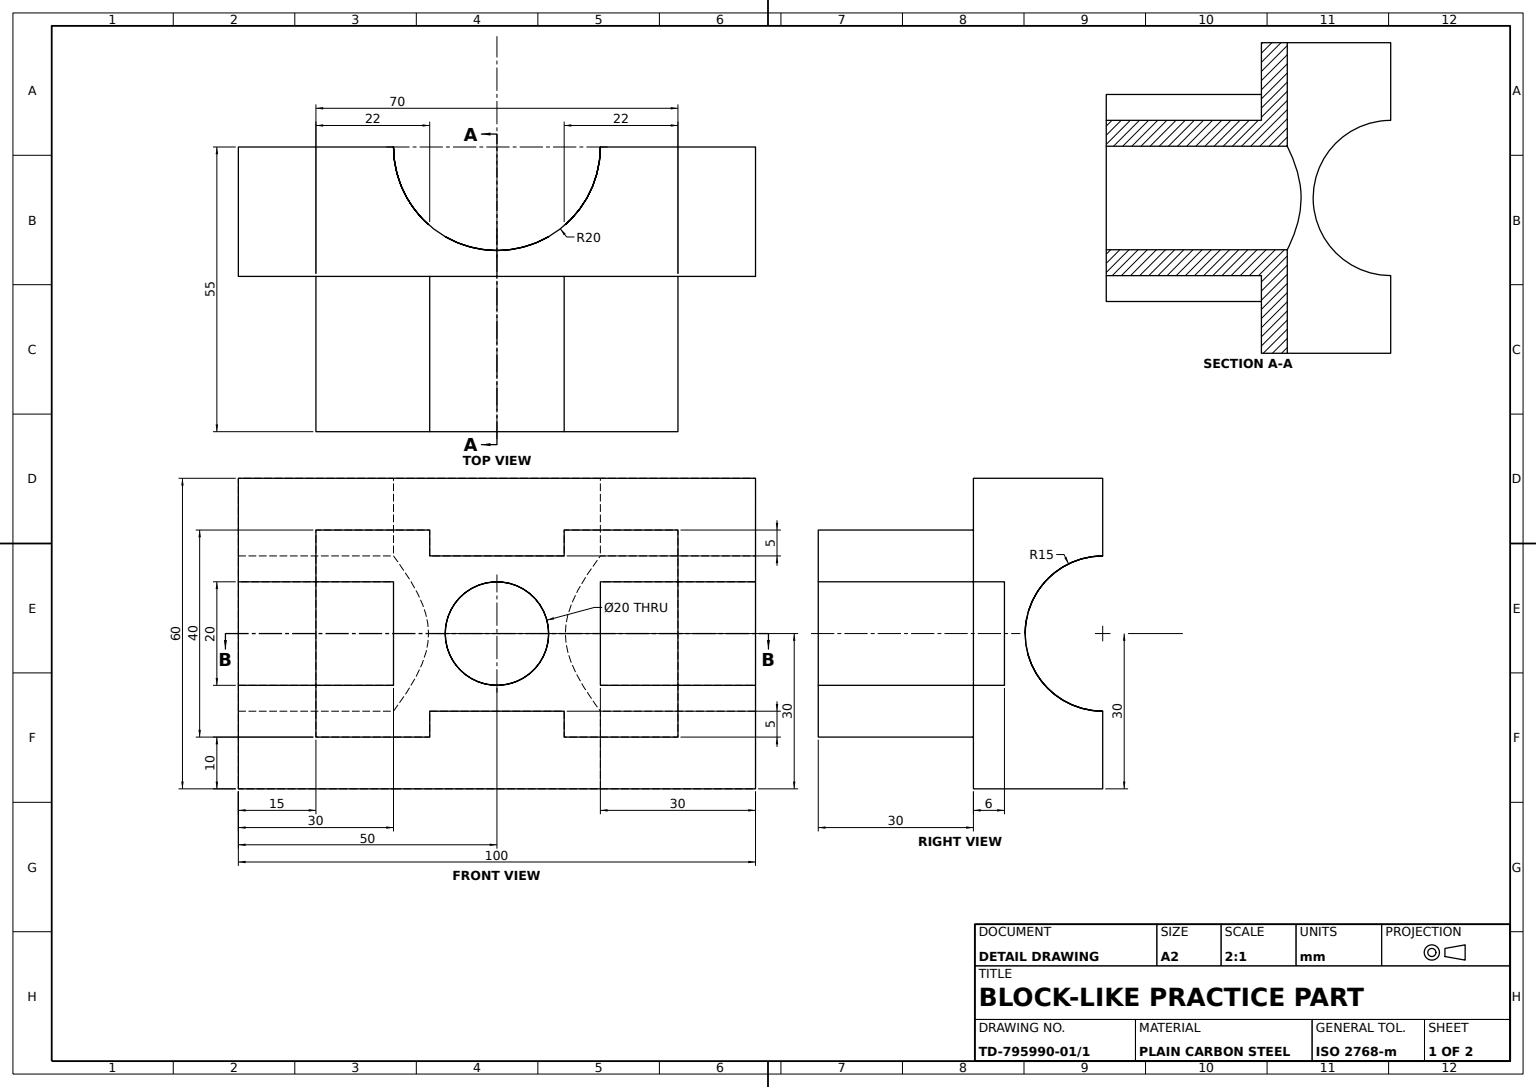
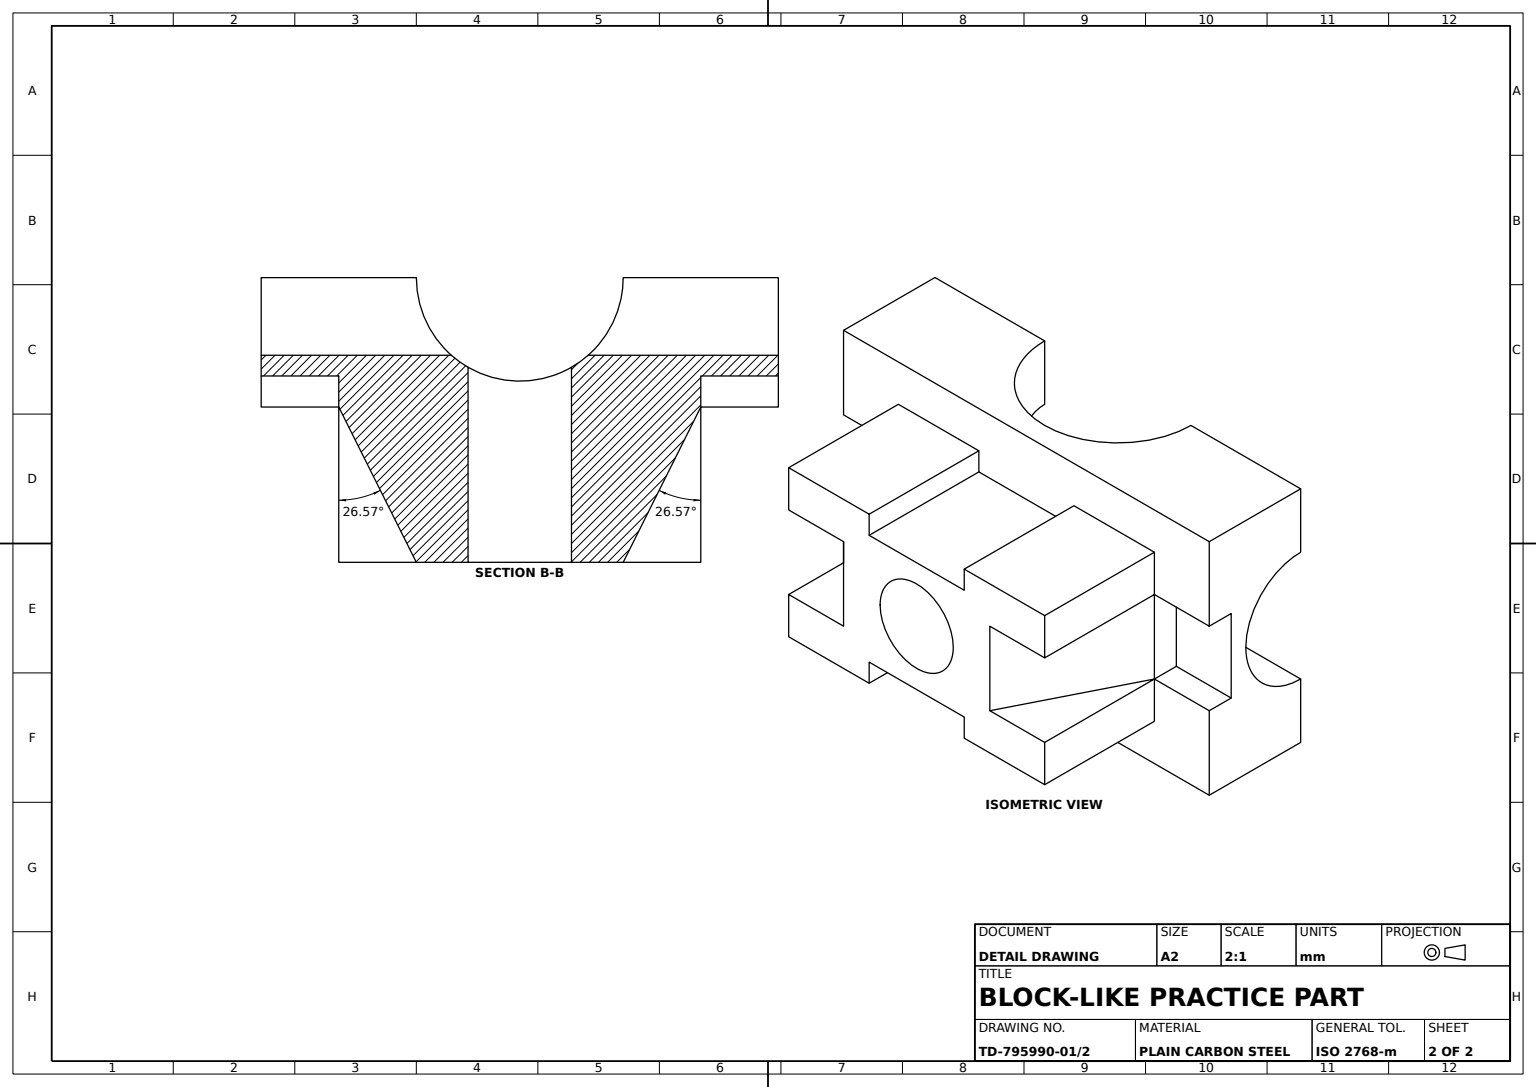
SolidWorks part; units mm, degrees
material "Plain Carbon Steel"
ref_plane "Front Plane" through (0, 0, 0) normal (0, 0, 1) x (1, 0, 0)
ref_plane "Top Plane" through (0, 0, 0) normal (0, 1, 0) x (1, 0, 0)
ref_plane "Right Plane" through (0, 0, 0) normal (1, 0, 0) x (0, 0, -1)
sketch "Base Plate Sketch" plane through (0, 0, 0) normal (0, 0, 1) x (1, 0, 0)
  line L0 (0, 0) -> (0, -60)
  line L1 (0, -60) -> (100, -60)
  line L2 (100, -60) -> (100, 0)
  line L3 (100, 0) -> (0, 0)
  dimension "D1" = 100
  dimension "D2" = 60
extrude "Base Plate 100x60x25" add sketch "Base Plate Sketch" along normal blind 25
sketch "T-Block Sketch" plane through (0, 0, 25) normal (0, 0, 1) x (1, 0, 0)
  line L0 (15, -10) -> (15, -50)
  line L1 (0, 0) -> (0, -60) construction
  line L3 (15, -10) -> (85, -10)
  line L4 (85, -10) -> (85, -50)
  line L5 (85, -50) -> (15, -50)
  line L6 (100, 0) -> (0, 0) construction
  dimension "D1" = 70
  dimension "D2" = 40
  dimension "D3" = 15
  dimension "D4" = 10
extrude "T-Block 70x40x30" add sketch "T-Block Sketch" along normal blind 30
sketch "Slot 15x20 Sketch" plane through (0, 0, 25) normal (0, 0, 1) x (1, 0, 0)
  line L0 (0, -20) -> (0, -40)
  line L1 (0, 0) -> (0, -60) construction
  line L2 (0, -20) -> (15, -20)
  line L3 (15, -40) -> (0, -40)
  line L4 (15, -20) -> (15, -40)
  line L5 (15, -10) -> (15, -50) construction
  dimension "D1" = 15
  dimension "D2" = 20
  dimension "D3" = 20
extrude "Slot 15x20 Depth 6" cut sketch "Slot 15x20 Sketch" against normal blind 6
sketch "Second Slot Sketch" plane through (0, 0, 25) normal (0, 0, 1) x (1, 0, 0)
  line L0 (100, -20) -> (100, -40)
  line L1 (100, -60) -> (100, 0) construction
  line L2 (100, -20) -> (85, -20)
  line L3 (85, -20) -> (85, -40)
  line L4 (85, -50) -> (85, -10) construction
  line L5 (85, -40) -> (100, -40)
  line L6 (15, -50) -> (85, -50) construction
  dimension "D1" = 10
  dimension "D2" = 30
extrude "Second Slot Depth 6" cut sketch "Second Slot Sketch" against normal blind 6
sketch "Side Arc Notch Sketch" plane through (0, -60, 0) normal (0, -1, 0) x (1, 0, 0)
  line L0 (0, 0) -> (100, 0) construction
  line L1 (30, 0) -> (70, 0)
  arc A0 (70, 0) -> (30, 0) centre (50, 0) ccw
  dimension "D1" = 20
extrude "Side Arc Notch" cut sketch "Side Arc Notch Sketch" against normal blind 60
sketch "End Arc Notch Sketch" plane through (0, 0, 0) normal (-1, 0, 0) x (0, 0, 1)
  line L0 (0, 0) -> (0, -60) construction
  line L1 (0, -15) -> (0, -45)
  arc A0 (0, -45) -> (0, -15) centre (0, -30) ccw
  dimension "D1" = 15
extrude "End Arc Notch" cut sketch "End Arc Notch Sketch" against normal blind 100
sketch "Block Recess A Sketch" plane through (0, 0, 55) normal (0, 0, 1) x (1, 0, 0)
  line L0 (37, -10) -> (63, -10)
  line L1 (85, -10) -> (15, -10) construction
  line L2 (85, -10) -> (15, -10) construction
  line L3 (37, -10) -> (37, -15)
  line L4 (37, -15) -> (63, -15)
  line L5 (63, -15) -> (63, -10)
  line L6 (15, -10) -> (15, -50) construction
  dimension "D1" = 22
  dimension "D2" = 48
  dimension "D3" = 5
extrude "Block Recess A" cut sketch "Block Recess A Sketch" against normal blind 30
sketch "Block Recess B Sketch" plane through (0, 0, 55) normal (0, 0, 1) x (1, 0, 0)
  line L0 (37, -50) -> (63, -50)
  line L1 (15, -50) -> (85, -50) construction
  line L2 (15, -50) -> (85, -50) construction
  line L3 (37, -50) -> (37, -45)
  line L4 (37, -45) -> (63, -45)
  line L5 (63, -45) -> (63, -50)
  line L6 (15, -10) -> (15, -50) construction
  line L7 (37, -10) -> (15, -10) construction
  dimension "D1" = 22
  dimension "D2" = 48
  dimension "D3" = 35
extrude "Block Recess B" cut sketch "Block Recess B Sketch" against normal blind 30
sketch "Cross Hole Sketch" plane through (0, 0, 55) normal (0, 0, 1) x (1, 0, 0)
  line L0 (85, -50) -> (85, -10) construction
  line L1 (63, -50) -> (85, -50) construction
  circle A0 centre (50, -30) radius 10
  dimension "D1" = 20
  dimension "D2" = 35
  dimension "D3" = 20
extrude "Cross Hole" cut sketch "Cross Hole Sketch" against normal blind 55
sketch "Wedge Cut A Sketch" plane through (0, -50, 0) normal (0, -1, 0) x (1, 0, 0)
  line L0 (15, 55) -> (30, 55)
  line L1 (15, 55) -> (37, 55) construction
  line L2 (30, 55) -> (15, 25)
  line L3 (15, 25) -> (15, 55)
  line L4 (37, 25) -> (37, 55) construction
  dimension "D1" = 7
extrude "Wedge Cut A" cut sketch "Wedge Cut A Sketch" against normal blind 30
sketch "Wedge Fill A Sketch" plane through (0, -50, 0) normal (0, -1, 0) x (1, 0, 0)
  line L0 (15, 25) -> (15, 55)
  line L1 (15, 55) -> (30, 55)
  line L2 (30, 55) -> (15, 25)
extrude "Wedge Fill A" add sketch "Wedge Fill A Sketch" against normal blind 10
sketch "Wedge Cut B Sketch" plane through (0, -50, 0) normal (0, -1, 0) x (1, 0, 0)
  line L0 (85, 55) -> (70, 55)
  line L1 (63, 55) -> (85, 55) construction
  line L2 (70, 55) -> (85, 25)
  line L3 (85, 25) -> (85, 55)
  line L4 (63, 25) -> (63, 55) construction
  dimension "D1" = 7
extrude "Wedge Cut B" cut sketch "Wedge Cut B Sketch" against normal blind 30
sketch "Wedge Fill B Sketch" plane through (0, -50, 0) normal (0, -1, 0) x (1, 0, 0)
  line L0 (70, 55) -> (85, 55)
  line L1 (85, 55) -> (85, 25)
  line L2 (85, 25) -> (70, 55)
extrude "Wedge Fill B" add sketch "Wedge Fill B Sketch" against normal blind 10
